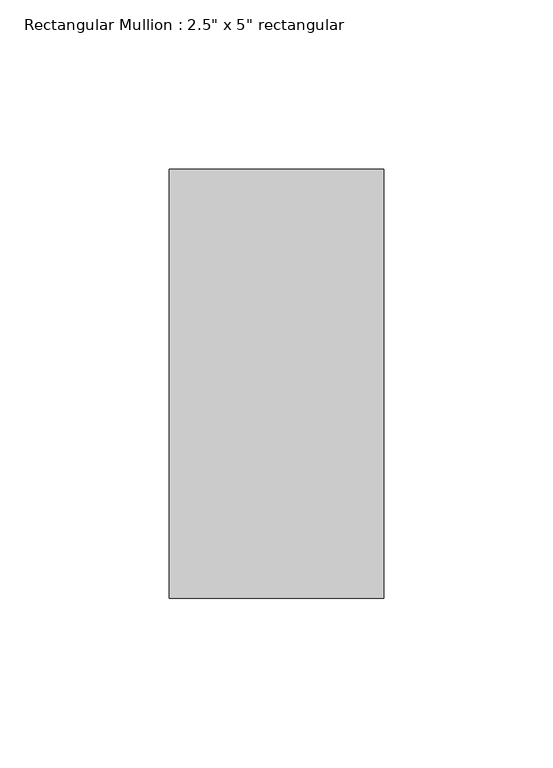
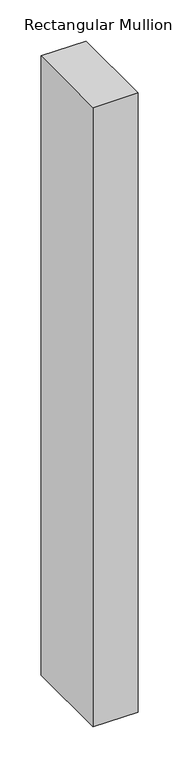
"""IFC4 building model written with IfcOpenShell, lengths in millimetres: member geometry."""

from ifc_helpers import new_model, si_unit, frame, origin, place, context, project, spatial, polyline, outline, extrude, source, transform, mapped, element, save


def member_5da52246(model_context):
    return source(origin(), model_context, "Body", "SweptSolid", [
        extrude(outline(polyline([(0.0, 63.5), (0.0, -63.5), (-63.5, -63.5), (-63.5, 63.5), (0.0, 63.5)])), frame((0.0, 0.0, -920.9617556), z_axis=(0.0, 0.0, 1.0), x_axis=(1.0, 0.0, 0.0)), (0.0, 0.0, 1.0), 920.9617556),
    ])


if __name__ == "__main__":
    model = new_model("IFC4")
    model_context = context("Model", 3, world=origin())
    ifc_project = project(units=[si_unit("LENGTHUNIT", "METRE", prefix="MILLI")], contexts=[model_context])
    site = spatial("IfcSite", under=ifc_project)
    building = spatial("IfcBuilding", under=site)
    placement = place(None, origin())
    member_shape = member_5da52246(model_context)
    element("IfcMember", 1, ObjectType="Rectangular Mullion : 2.5\" x 5\" rectangular", at=placement, inside=building, context=model_context, shape_type="MappedRepresentation", body=[
        mapped(member_shape, transform((0.0, 0.0, 0.0), x_axis=(1.0, 0.0, 0.0), y_axis=(0.0, 1.0, 0.0), z_axis=(0.0, 0.0, 1.0))),
    ])
    save(model, "model.ifc")

# Revit data of these elements
# Type "Rectangular Mullion : 2.5\" x 5\" rectangular"
#   built-in parameter 1007304 = 0.416667 (stored number, unit not read)
#   built-in parameter 1007301 = 0.104167 (stored number, unit not read)
#   built-in parameter 1007300 = 0.104167 (stored number, unit not read)
# Element 1 (IfcMember, "Rectangular Mullion : 2.5\" x 5\" rectangular")
#   Materials on its faces: "Aluminum"
# Materials
#   "Aluminum": class "Metal", colour RGB 247 247 247, transparency 0, Description = "Aluminum 6061", Cost = 0
